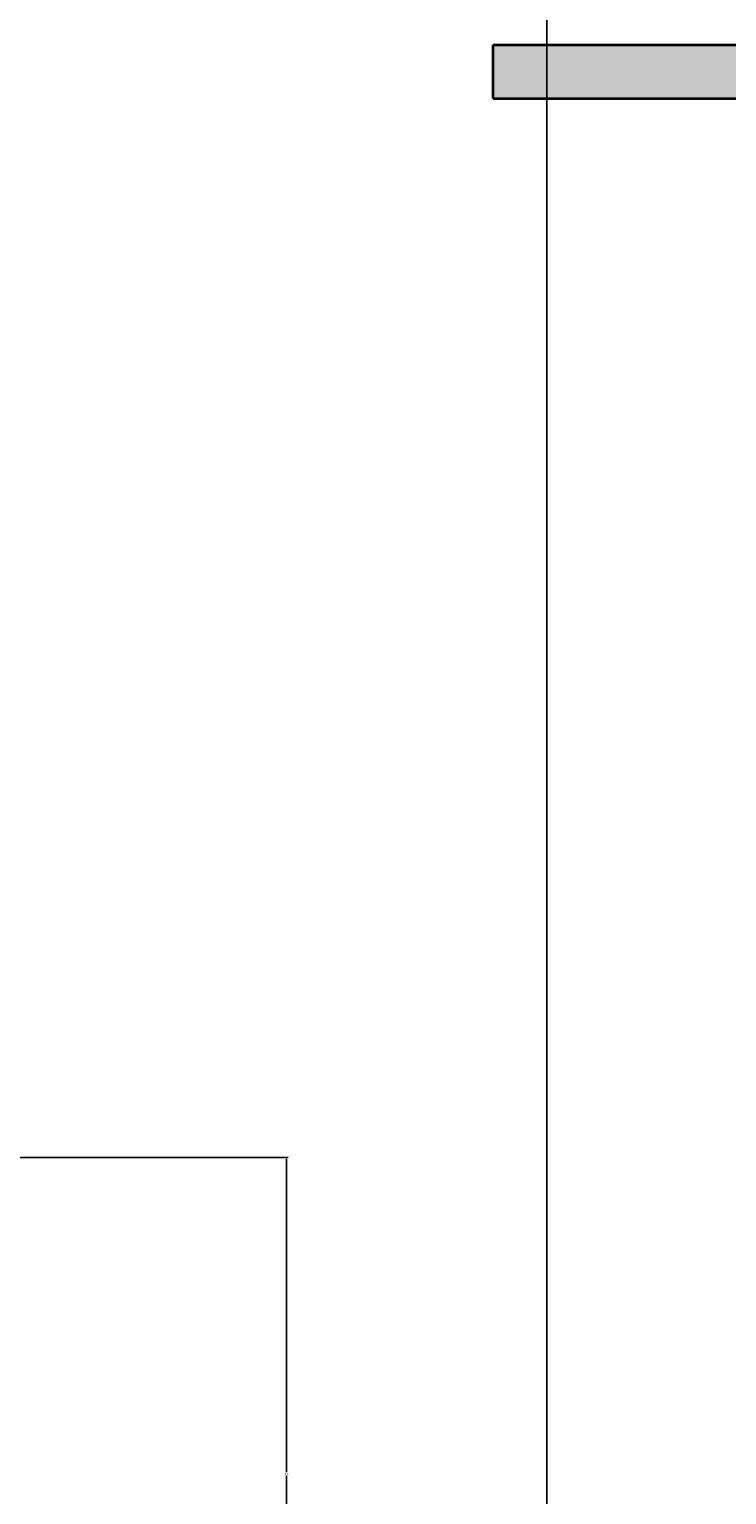
# Model space of a CAD drawing. Units: inches. Extents: x 2549 to 3108, y 1683 to 2362.
# Tile 18 of 30: x 2815 to 2893, y 1979 to 2142. Entities that reach past the tile are written whole.
import ezdxf

# ---------------------------------------------------------------- set-up
doc = ezdxf.new("R2010")
doc.units = ezdxf.units.IN
for name, color, linetype, lineweight in [('A-ANNO-DIMS', 2, 'Continuous', 18), ('A-WALL', 7, 'Continuous', 35), ('A-WALL-PATT', 89, 'Continuous', 13)]:
    doc.layers.add(name, color=color, linetype=linetype, lineweight=lineweight)
doc.layers.add('C-PKNG-VEHI-PATT', color=251, linetype='Continuous', lineweight=13, true_color=0x636466)
doc.layers.add('C-PVMT-PATT', color=9, linetype='Continuous', lineweight=13, true_color=0xc7c8ca)
doc.styles.get("Standard").update_dxf_attribs({"font": 'arial.ttf'})
doc.dimstyles.get("Standard").update_dxf_attribs({"dimtxt": 0.18, "dimasz": 0.18, "dimexe": 0.18, "dimexo": 0.0625, "dimgap": 0.09, "dimtad": 0, "dimtih": 1, "dimtoh": 1, "dimdec": 4, "dimzin": 0, "dimdsep": 46, "dimtxsty": 'Standard', "dimcen": 0.09, "dimadec": 0, "dimazin": 0, "dimtfac": 1, "dimtdec": 4, "dimtofl": 0, "dimtmove": 0, "dimatfit": 3, "dimfxl": 1, "dimtolj": 1, "dimtzin": 0, "dimarcsym": 0})

# ---------------------------------------------------------------- blocks, each defined once
blk = doc.blocks.new('*D46')
at = {"layer": 'A-ANNO-DIMS', "color": 0, "lineweight": -2, "transparency": 16777216}
for p, q in [((2812.64, 2140.46), (2812.64, 1683.44)), ((3034.64, 2134.46), (3034.64, 1683.44)), ((2812.82, 1683.62), (2923.35, 1683.62)), ((3034.46, 1683.62), (2923.93, 1683.62))]:
    blk.add_line(p, q, dxfattribs=at)
at = {"layer": 'A-ANNO-DIMS', "color": 0, "transparency": 16777216}
for points in [[(2812.82, 1683.65), (2812.82, 1683.59), (2812.64, 1683.62)], [(3034.46, 1683.65), (3034.46, 1683.59), (3034.64, 1683.62)]]:
    blk.add_solid(points, dxfattribs=at)
at = {"layer": 'Defpoints', "color": 0, "transparency": 16777216}
for p in [(2812.64, 2140.52), (3034.64, 2134.52), (3034.64, 1683.62)]:
    blk.add_point(p, dxfattribs=at)
at = {"layer": 'A-ANNO-DIMS', "color": 0, "transparency": 16777216, "insert": (2923.64, 1683.62), "char_height": 0.18, "attachment_point": 5}
blk.add_mtext('\\A1;222', dxfattribs=at)
blk = doc.blocks.new('*D48')
at = {"layer": 'A-ANNO-DIMS', "color": 0, "lineweight": -2, "transparency": 16777216}
for p, q in [((2812.71, 2016.19), (2843.72, 2016.19)), ((2843.54, 2016.01), (2843.54, 1981.04)), ((2843.54, 1945.7), (2843.54, 1980.68)), ((2812.71, 1945.52), (2843.72, 1945.52))]:
    blk.add_line(p, q, dxfattribs=at)
at = {"layer": 'A-ANNO-DIMS', "color": 0, "transparency": 16777216}
for points in [[(2843.51, 2016.01), (2843.57, 2016.01), (2843.54, 2016.19)], [(2843.51, 1945.7), (2843.57, 1945.7), (2843.54, 1945.52)]]:
    blk.add_solid(points, dxfattribs=at)
at = {"layer": 'Defpoints', "color": 0, "transparency": 16777216}
for p in [(2812.64, 2016.19), (2812.64, 1945.52), (2843.54, 1945.52)]:
    blk.add_point(p, dxfattribs=at)
at = {"layer": 'A-ANNO-DIMS', "color": 0, "transparency": 16777216, "insert": (2843.54, 1980.86), "char_height": 0.18, "attachment_point": 5}
blk.add_mtext('\\A1;70.67', dxfattribs=at)
blk = doc.blocks.new('*D52')
at = {"layer": 'A-ANNO-DIMS', "color": 0, "lineweight": -2, "transparency": 16777216}
for p, q in [((2812.64, 1891.59), (2812.64, 2362.32)), ((2812.82, 2362.14), (2842.42, 2362.14)), ((2872.46, 2362.14), (2842.86, 2362.14)), ((2872.64, 1891.59), (2872.64, 2362.32))]:
    blk.add_line(p, q, dxfattribs=at)
at = {"layer": 'A-ANNO-DIMS', "color": 0, "transparency": 16777216}
for points in [[(2812.82, 2362.17), (2812.82, 2362.11), (2812.64, 2362.14)], [(2872.46, 2362.17), (2872.46, 2362.11), (2872.64, 2362.14)]]:
    blk.add_solid(points, dxfattribs=at)
at = {"layer": 'Defpoints', "color": 0, "transparency": 16777216}
for p in [(2872.64, 2362.14), (2812.64, 1891.52), (2872.64, 1891.52)]:
    blk.add_point(p, dxfattribs=at)
at = {"layer": 'A-ANNO-DIMS', "color": 0, "transparency": 16777216, "insert": (2842.64, 2362.14), "char_height": 0.18, "attachment_point": 5}
blk.add_mtext('\\A1;60', dxfattribs=at)

msp = doc.modelspace()

# ---------------------------------------------------------------- hatches: boundary and pattern name
at = {"layer": 'A-WALL-PATT'}
h = msp.add_hatch(color=256, dxfattribs=at)
h.dxf.hatch_style = 1
h.paths.add_polyline_path([(2812.6427, 2272.5237), (2806.6427, 2272.5237), (2806.6427, 2182.5237), (2815.3646, 2182.5237), (2815.3646, 2188.5237), (2812.6427, 2188.5237)])
h.paths.add_polyline_path([(2872.6427, 2272.5237), (2866.6427, 2272.5237), (2866.6427, 2188.5237), (2837.9934, 2188.5237), (2837.9934, 2182.5237), (2872.6427, 2182.5237)])
h.paths.add_polyline_path([(3034.6427, 2140.5237), (2866.6427, 2140.5237), (2866.6427, 2134.5237), (3034.6427, 2134.5237)])
at = {"layer": 'C-PKNG-VEHI-PATT'}
h = msp.add_hatch(color=256, dxfattribs=at)
h.dxf.hatch_style = 1
edge = h.paths.add_edge_path()
edge.add_ellipse((2935.7258, 1791.964), major_axis=(-50.66, 0), ratio=0.84230387, start_angle=248.165046, end_angle=265.722579)
edge.add_line((2938.911, 1834.5507), (2925.8653, 1834.5507))
edge.add_ellipse((2929.0505, 1791.964), major_axis=(50.66, 0), ratio=0.84230387, start_angle=94.277421, end_angle=111.834954)
edge.add_line((2912.8508, 1832.3947), (2914.2044, 1822.2495))
edge.add_ellipse((2930.6538, 1783.1023), major_axis=(-49.3014, 0), ratio=0.84230387, start_angle=-85.12993, end_angle=-67.208085, ccw=False)
edge.add_line((2927.1247, 1824.5225), (2937.6516, 1824.5225))
edge.add_ellipse((2934.1225, 1783.1023), major_axis=(49.3014, 0), ratio=0.84230387, start_angle=67.208085, end_angle=85.12993, ccw=False)
edge.add_line((2950.5719, 1822.2495), (2951.9255, 1832.3947))
edge = h.paths.add_edge_path()
edge.add_ellipse((2903.4793, 1857.3351), major_axis=(-34.7979, 0), ratio=0.84230387, start_angle=180, end_angle=209.43857)
edge.add_ellipse((2961.297, 1857.3351), major_axis=(34.7979, 0), ratio=0.84230387, start_angle=150.56143, end_angle=180)
edge.add_line((2926.4991, 1857.3351), (2926.4991, 1843.7609))
edge.add_ellipse((2924.1251, 1844.3143), major_axis=(-0.2209, 3.9278), ratio=0.60383358, start_angle=89.002014, end_angle=253.657408, ccw=False)
edge.add_line((2921.7512, 1844.2222), (2921.7512, 1853.3975))
edge.add_line((2921.7512, 1853.3975), (2925.269, 1855.8484))
edge.add_ellipse((2925.4782, 1855.4931), major_axis=(0.4584, 0), ratio=0.84230387, start_angle=90, end_angle=134.480211, ccw=False)
edge.add_line((2925.4782, 1855.8792), (2926.4991, 1855.8792))
edge.add_line((2926.4991, 1855.8792), (2926.4991, 1857.3351))
edge.add_ellipse((2961.297, 1857.3351), major_axis=(34.7979, 0), ratio=0.84230387, start_angle=150.56143, end_angle=180, ccw=False)
edge.add_line((2932.3882, 1873.6501), (2932.3882, 1875.7801))
edge.add_ellipse((2932.3882, 1875.3939), major_axis=(0.4584, 0), ratio=0.84230387, start_angle=90, end_angle=127.93313)
edge.add_line((2932.1366, 1875.7167), (2928.5915, 1873.7564))
edge.add_ellipse((2899.9271, 2002.4692), major_axis=(155.4756, 0), ratio=0.84230387, start_angle=-80.743434, end_angle=-77.445067, ccw=False)
edge.add_ellipse((2949.4402, 1715.2151), major_axis=(-189.1422, 0), ratio=0.84230387, start_angle=-79.790461, end_angle=-77.555373)
edge.add_ellipse((3300.3614, 1852.5642), major_axis=(-386.1662, 0), ratio=0.84230387, start_angle=-2.863715, end_angle=2.198541)
edge.add_ellipse((2929.0505, 1792.5159), major_axis=(-55.6192, 0), ratio=0.84230387, start_angle=-85.917589, end_angle=-72.280047, ccw=False)
edge.add_line((2925.7129, 1839.2798), (2939.0634, 1839.2798))
edge.add_ellipse((2935.7258, 1792.5159), major_axis=(55.6192, 0), ratio=0.84230387, start_angle=72.280047, end_angle=85.917589, ccw=False)
edge.add_ellipse((2564.4149, 1852.5642), major_axis=(-386.1662, 0), ratio=0.84230387, start_angle=177.801459, end_angle=182.863715)
edge.add_ellipse((2915.3361, 1715.2151), major_axis=(189.1422, 0), ratio=0.84230387, start_angle=77.555373, end_angle=79.790461)
edge.add_ellipse((2964.8492, 2002.4692), major_axis=(-155.4756, 0), ratio=0.84230387, start_angle=77.445067, end_angle=80.743434, ccw=False)
edge.add_line((2936.1848, 1873.7564), (2932.6397, 1875.7167))
edge.add_ellipse((2932.3882, 1875.3939), major_axis=(0.4584, 0), ratio=0.84230387, start_angle=52.06687, end_angle=90)
edge.add_line((2932.3882, 1875.7801), (2932.3882, 1873.6501))
edge.add_ellipse((2903.4793, 1857.3351), major_axis=(-34.7979, 0), ratio=0.84230387, start_angle=180, end_angle=209.43857, ccw=False)
edge.add_line((2938.2772, 1857.3351), (2938.2772, 1855.8792))
edge.add_line((2938.2772, 1855.8792), (2939.4059, 1855.8792))
edge.add_ellipse((2939.2981, 1855.4931), major_axis=(-0.4584, 0), ratio=0.84230387, start_angle=225.519789, end_angle=270, ccw=False)
edge.add_line((2939.5903, 1855.7906), (2943.0251, 1853.3975))
edge.add_line((2943.0251, 1853.3975), (2943.0251, 1844.2222))
edge.add_ellipse((2940.6512, 1844.3143), major_axis=(0.2209, 3.9278), ratio=0.60383358, start_angle=106.342592, end_angle=270.997986, ccw=False)
edge.add_line((2938.2772, 1843.7609), (2938.2772, 1857.3351))
edge = h.paths.add_edge_path()
edge.add_ellipse((2932.3882, 1865.1973), major_axis=(91.081, 0), ratio=0.84230387, start_angle=256.401865, end_angle=283.598135, ccw=False)
edge.add_line((2914.2044, 1790.0239), (2914.2044, 1778.3622))
edge.add_ellipse((2932.3882, 1853.5356), major_axis=(91.081, 0), ratio=0.84230387, start_angle=256.401865, end_angle=283.598135)
edge.add_line((2950.5719, 1778.3622), (2950.5719, 1790.0239))
edge = h.paths.add_edge_path()
edge.add_ellipse((2948.7383, 1772.3145), major_axis=(1.8336, 0), ratio=0.84230387, start_angle=0, end_angle=90)
edge.add_line((2948.7383, 1773.859), (2916.038, 1773.859))
edge.add_ellipse((2916.038, 1772.3145), major_axis=(1.8336, 0), ratio=0.84230387, start_angle=90, end_angle=180)
edge.add_line((2914.2044, 1772.3145), (2914.2044, 1760.2558))
edge.add_line((2914.2044, 1760.2558), (2950.5719, 1760.2558))
edge.add_line((2950.5719, 1760.2558), (2950.5719, 1772.3145))
h.paths.add_polyline_path([(2748.8496, 2101.6383), (2798.148, 2101.6383), (2798.148, 2111.4248), (2748.8496, 2111.4248)], flags=9)
h.paths.add_polyline_path([(2685.2081, 2101.489), (2719.3253, 2101.489), (2719.3253, 2111.2819), (2685.2081, 2111.2819)], flags=9)
h.paths.add_polyline_path([(2814.6852, 1907.1328), (2847.8384, 1907.1328), (2847.8384, 1916.9258), (2814.6852, 1916.9258)], flags=9)
h.paths.add_polyline_path([(2814.3906, 1835.5864), (2848.0172, 1835.5864), (2848.0172, 1845.3794), (2814.3906, 1845.3794)], flags=9)
h.paths.add_polyline_path([(2800.5245, 1759.1674), (2853.7435, 1759.1674), (2853.7435, 1768.954), (2800.5245, 1768.954)], flags=9)
h.paths.add_polyline_path([(2972.4611, 1807.3305), (3015.3943, 1807.3305), (3015.3943, 1817.117), (2972.4611, 1817.117)], flags=9)
h.paths.add_polyline_path([(2902.3327, 1888.6731), (2937.9131, 1888.6731), (2937.9131, 1898.4661), (2902.3327, 1898.4661)], flags=9)
h.paths.add_polyline_path([(2712.1779, 1878.9039), (2754.1257, 1878.9039), (2754.1257, 1888.6904), (2712.1779, 1888.6904)], flags=9)
h.paths.add_polyline_path([(2614.0056, 2012.812), (2650.0251, 2012.812), (2650.0251, 2022.4371), (2614.0056, 2022.4371)], flags=9)
h.paths.add_polyline_path([(2713.3129, 2003.1645), (2747.4237, 2003.1645), (2747.4237, 2012.951), (2713.3129, 2012.951)], flags=9)
h.paths.add_polyline_path([(2950.1379, 2001.6934), (2982.2992, 2001.6934), (2982.2992, 2011.48), (2950.1379, 2011.48)], flags=9)
h.paths.add_polyline_path([(2940.864, 2238.5537), (2997.5066, 2238.5537), (2997.5066, 2248.3466), (2940.864, 2248.3466)], flags=9)
h.paths.add_polyline_path([(2821.5457, 2202.8348), (2855.663, 2202.8348), (2855.663, 2212.6278), (2821.5457, 2212.6278)], flags=9)
h.paths.add_polyline_path([(2661.8026, 2238.6249), (2718.4451, 2238.6249), (2718.4451, 2248.4179), (2661.8026, 2248.4179)], flags=9)
at = {"layer": 'C-PVMT-PATT'}
h = msp.add_hatch(color=256, dxfattribs=at)
h.dxf.hatch_style = 1
h.paths.add_polyline_path([(3067.6427, 2305.5237), (2605.6427, 2305.5237), (2605.6427, 2074.5237), (2629.6427, 2074.5237), (2629.6427, 2281.5237), (3043.6427, 2281.5237), (3043.6427, 1885.5237), (3043.6427, 1872.8745), (3031.1672, 1872.8745), (3031.1672, 1862.5731), (2995.8054, 1862.5731), (2995.8054, 1872.8745), (2983.1752, 1872.8745), (2983.1752, 1885.5237), (2881.6427, 1885.5237), (2881.6427, 1795.5237), (2751.0977, 1795.5237), (2751.0977, 1761.5237), (2786.1577, 1761.5237), (2786.1577, 1723.5237), (2881.84, 1723.5237), (2881.84, 1714.5237), (3067.6427, 1714.5237), (3067.6427, 1723.5237)])
edge = h.paths.add_edge_path(flags=16)
edge.add_ellipse((2949.4402, 1710.9683), major_axis=(-194.1014, 0), ratio=0.84230387, start_angle=-77.874034, end_angle=-76.219471, ccw=False)
edge.add_ellipse((2949.4402, 1715.2151), major_axis=(-189.1422, 0), ratio=0.84230387, start_angle=-79.790461, end_angle=-77.555373, ccw=False)
edge.add_ellipse((2899.9271, 2002.4692), major_axis=(155.4756, 0), ratio=0.84230387, start_angle=-80.743434, end_angle=-77.445067)
edge.add_line((2928.5915, 1873.7564), (2932.3882, 1875.8558))
edge.add_line((2932.3882, 1875.8558), (2936.1848, 1873.7564))
edge.add_ellipse((2964.8492, 2002.4692), major_axis=(-155.4756, 0), ratio=0.84230387, start_angle=77.445067, end_angle=80.743434)
edge.add_ellipse((2915.3361, 1715.2151), major_axis=(189.1422, 0), ratio=0.84230387, start_angle=77.555373, end_angle=79.790461, ccw=False)
edge.add_ellipse((2915.3361, 1710.9683), major_axis=(-194.1014, 0), ratio=0.84230387, start_angle=256.219471, end_angle=257.874034, ccw=False)
edge.add_ellipse((2628.2871, 1850.2612), major_axis=(-327.2532, 0), ratio=0.84230387, start_angle=182.17995, end_angle=183.650428, ccw=False)
edge.add_ellipse((2955.5637, 1861.9334), major_axis=(-0.9168, 0), ratio=0.84230387, start_angle=180, end_angle=270, ccw=False)
edge.add_line((2956.4805, 1862.3857), (2956.4805, 1846.4866))
edge.add_ellipse((2955.5637, 1846.939), major_axis=(-0.9168, 0), ratio=0.84230387, start_angle=90, end_angle=180, ccw=False)
edge.add_ellipse((-3607.0606, 1835.832), major_axis=(-6562.6242, 0), ratio=0.84230387, start_angle=179.61613322, end_angle=180.09022909, ccw=False)
edge.add_ellipse((2955.5637, 1791.0926), major_axis=(0.9168, 0), ratio=0.84230387, start_angle=0, end_angle=90, ccw=False)
edge.add_line((2956.4805, 1791.545), (2956.4805, 1775.6459))
edge.add_ellipse((2955.5637, 1776.0982), major_axis=(0.9168, 0), ratio=0.84230387, start_angle=270, end_angle=360, ccw=False)
edge.add_ellipse((-3607.0606, 1835.832), major_axis=(-6562.6242, 0), ratio=0.84230387, start_angle=179.3813568, end_angle=179.47172853, ccw=False)
edge.add_ellipse((2954.5907, 1763.8768), major_axis=(-1.3752, 0), ratio=0.84230387, start_angle=179.371763, end_angle=248.464757, ccw=False)
edge.add_ellipse((-3607.519, 1835.832), major_axis=(-6564.0409, 0), ratio=0.842303863, start_angle=179.35344594, end_angle=179.37176282, ccw=False)
edge.add_ellipse((2952.6829, 1761.8002), major_axis=(3.2503, 0), ratio=0.84230387, start_angle=-90, end_angle=-0.646554, ccw=False)
edge.add_line((2952.6829, 1759.0625), (2912.0934, 1759.0625))
edge.add_ellipse((2912.0934, 1761.8002), major_axis=(3.2503, 0), ratio=0.84230387, start_angle=180.646554, end_angle=270, ccw=False)
edge.add_ellipse((9472.2953, 1835.832), major_axis=(-6564.0409, 0), ratio=0.842303871, start_angle=0.62823722, end_angle=0.6465541, ccw=False)
edge.add_ellipse((2910.1856, 1763.8768), major_axis=(1.3752, 0), ratio=0.84230387, start_angle=111.535244, end_angle=180.628237, ccw=False)
edge.add_ellipse((9471.8369, 1835.832), major_axis=(-6562.6242, 0), ratio=0.84230387, start_angle=0.52827147, end_angle=0.6465541, ccw=False)
edge.add_ellipse((2909.2126, 1776.0982), major_axis=(-0.9168, 0), ratio=0.84230387, start_angle=0, end_angle=90, ccw=False)
edge.add_line((2908.2958, 1775.6459), (2908.2958, 1791.545))
edge.add_ellipse((2909.2126, 1791.0926), major_axis=(-0.9168, 0), ratio=0.84230387, start_angle=-90, end_angle=0, ccw=False)
edge.add_ellipse((9471.8369, 1835.832), major_axis=(-6562.6242, 0), ratio=0.84230387, start_angle=-0.09022909, end_angle=0.38386678, ccw=False)
edge.add_ellipse((2909.2126, 1846.939), major_axis=(-0.9168, 0), ratio=0.84230387, start_angle=0, end_angle=90, ccw=False)
edge.add_line((2908.2958, 1846.4866), (2908.2958, 1862.3857))
edge.add_ellipse((2909.2126, 1861.9334), major_axis=(0.9168, 0), ratio=0.84230387, start_angle=90, end_angle=180, ccw=False)
edge.add_ellipse((3236.4892, 1850.2612), major_axis=(327.2532, 0), ratio=0.84230387, start_angle=176.349572, end_angle=177.82005, ccw=False)
edge = h.paths.add_edge_path(flags=0)
edge.add_ellipse((2903.4793, 1857.3351), major_axis=(-34.7979, 0), ratio=0.84230387, start_angle=180, end_angle=209.43857, ccw=False)
edge.add_line((2938.2772, 1857.3351), (2938.2772, 1855.8792))
edge.add_line((2938.2772, 1855.8792), (2939.4631, 1855.8792))
edge.add_line((2939.4631, 1855.8792), (2943.0251, 1853.3975))
edge.add_line((2943.0251, 1853.3975), (2943.0251, 1844.2222))
edge.add_ellipse((2940.6512, 1844.3143), major_axis=(0.2209, 3.9278), ratio=0.60383358, start_angle=106.342592, end_angle=270.997986, ccw=False)
edge.add_line((2938.2772, 1843.7609), (2938.2772, 1857.3351))
edge.add_ellipse((2903.4793, 1857.3351), major_axis=(-34.7979, 0), ratio=0.84230387, start_angle=180, end_angle=209.43857)
edge.add_ellipse((2961.297, 1857.3351), major_axis=(34.7979, 0), ratio=0.84230387, start_angle=150.56143, end_angle=180)
edge.add_line((2926.4991, 1857.3351), (2926.4991, 1843.7609))
edge.add_ellipse((2924.1251, 1844.3143), major_axis=(-0.2209, 3.9278), ratio=0.60383358, start_angle=89.002014, end_angle=253.657408, ccw=False)
edge.add_line((2921.7512, 1844.2222), (2921.7512, 1853.3975))
edge.add_line((2921.7512, 1853.3975), (2925.3132, 1855.8792))
edge.add_line((2925.3132, 1855.8792), (2926.4991, 1855.8792))
edge.add_line((2926.4991, 1855.8792), (2926.4991, 1857.3351))
edge.add_ellipse((2961.297, 1857.3351), major_axis=(34.7979, 0), ratio=0.84230387, start_angle=150.56143, end_angle=180, ccw=False)
edge = h.paths.add_edge_path(flags=0)
edge.add_ellipse((2929.0505, 1791.964), major_axis=(50.66, 0), ratio=0.84230387, start_angle=94.277421, end_angle=111.834954, ccw=False)
edge.add_line((2925.8653, 1834.5507), (2938.911, 1834.5507))
edge.add_ellipse((2935.7258, 1791.964), major_axis=(-50.66, 0), ratio=0.84230387, start_angle=248.165046, end_angle=265.722579, ccw=False)
edge.add_line((2951.9255, 1832.3947), (2950.5719, 1822.2495))
edge.add_ellipse((2934.1225, 1783.1023), major_axis=(49.3014, 0), ratio=0.84230387, start_angle=67.208085, end_angle=85.12993)
edge.add_line((2937.6516, 1824.5225), (2927.1247, 1824.5225))
edge.add_ellipse((2930.6538, 1783.1023), major_axis=(-49.3014, 0), ratio=0.84230387, start_angle=-85.12993, end_angle=-67.208085)
edge.add_line((2914.2044, 1822.2495), (2912.8508, 1832.3947))
edge = h.paths.add_edge_path(flags=0)
edge.add_line((2910.1338, 1829.4651), (2912.6432, 1821.2711))
edge.add_ellipse((5203.7787, 1816.4367), major_axis=(-2291.1426, 0), ratio=0.84230387, start_angle=-0.1208974, end_angle=0.3640763)
edge.add_line((2912.7012, 1801.8782), (2910.3305, 1792.5698))
edge.add_ellipse((9471.8369, 1835.832), major_axis=(-6561.7074, 0), ratio=0.84230387, start_angle=0.05559431, end_angle=0.37776419, ccw=False)
edge = h.paths.add_edge_path(flags=0)
edge.add_ellipse((-3607.0606, 1835.832), major_axis=(6561.7074, 0), ratio=0.84230387, start_angle=-0.37776419, end_angle=-0.05559431, ccw=False)
edge.add_line((2954.4458, 1792.5698), (2952.0751, 1801.8782))
edge.add_ellipse((660.9976, 1816.4367), major_axis=(2291.1426, 0), ratio=0.84230387, start_angle=-0.3640763, end_angle=0.1208974)
edge.add_line((2952.1331, 1821.2711), (2954.6425, 1829.4651))
edge = h.paths.add_edge_path(flags=0)
edge.add_ellipse((2932.3882, 1865.1973), major_axis=(91.081, 0), ratio=0.84230387, start_angle=256.401865, end_angle=283.598135)
edge.add_line((2950.5719, 1790.0239), (2950.5719, 1778.3622))
edge.add_ellipse((2932.3882, 1853.5356), major_axis=(91.081, 0), ratio=0.84230387, start_angle=256.401865, end_angle=283.598135, ccw=False)
edge.add_line((2914.2044, 1778.3622), (2914.2044, 1790.0239))
edge = h.paths.add_edge_path(flags=0)
edge.add_line((2916.038, 1773.859), (2948.7383, 1773.859))
edge.add_ellipse((2948.7383, 1772.3145), major_axis=(1.8336, 0), ratio=0.84230387, start_angle=0, end_angle=90, ccw=False)
edge.add_line((2950.5719, 1772.3145), (2950.5719, 1760.2558))
edge.add_line((2950.5719, 1760.2558), (2914.2044, 1760.2558))
edge.add_line((2914.2044, 1760.2558), (2914.2044, 1772.3145))
edge.add_ellipse((2916.038, 1772.3145), major_axis=(1.8336, 0), ratio=0.84230387, start_angle=90, end_angle=180, ccw=False)
h.paths.add_polyline_path([(2629.6427, 1978.5237), (2605.6427, 1978.5237), (2605.6427, 1723.5237), (2629.6427, 1723.5237), (2629.6427, 1795.5237)], flags=17)
h.paths.add_polyline_path([(2800.5245, 1759.1674), (2853.7435, 1759.1674), (2853.7435, 1768.954), (2800.5245, 1768.954)], flags=24)
h.paths.add_polyline_path([(2972.4611, 1807.3305), (3015.3943, 1807.3305), (3015.3943, 1817.117), (2972.4611, 1817.117)], flags=24)

# ---------------------------------------------------------------- linework, layer by layer
at = {"layer": 'A-WALL'}
for p, q in [((2866.6427, 2134.5237), (2866.6427, 2140.5237)), ((2866.6427, 2140.5237), (3034.6427, 2140.5237)), ((2866.6427, 2134.5237), (3034.6427, 2134.5237))]:
    msp.add_line(p, q, dxfattribs=at)

# ---------------------------------------------------------------- dimensions: what is measured, and where the dimension line sits
at = {"layer": 'A-ANNO-DIMS'}
for base, p1, p2, picture, middle in [((2872.6427, 2362.1425), (2812.6427, 1891.5237), (2872.6427, 1891.5237), '*D52', (2842.6427, 2362.1425)), ((3034.6427, 1683.6237), (2812.6427, 2140.5237), (3034.6427, 2134.5237), '*D46', (2923.6427, 1683.6237))]:
    dim = msp.add_linear_dim(base=base, p1=p1, p2=p2, dimstyle='Standard', override={"dimdec": 0, "dimlfac": 1, "dimrnd": 0, "dimzin": 0, "dimdsep": 46, "dimlunit": 2}, dxfattribs=at)
    dim.commit()
    dim.dimension.update_dxf_attribs({"geometry": picture, "text_midpoint": middle})
dim = msp.add_linear_dim(base=(2843.5427, 1945.5237), p1=(2812.6427, 2016.1911), p2=(2812.6427, 1945.5237), angle=270, dimstyle='Standard', override={"dimdec": 2, "dimlfac": 1, "dimrnd": 0, "dimzin": 0, "dimdsep": 46, "dimlunit": 2}, dxfattribs=at)
dim.commit()
dim.dimension.update_dxf_attribs({"geometry": '*D48', "text_midpoint": (2843.5427, 1980.8574)})

doc.saveas('drawing.dxf')
